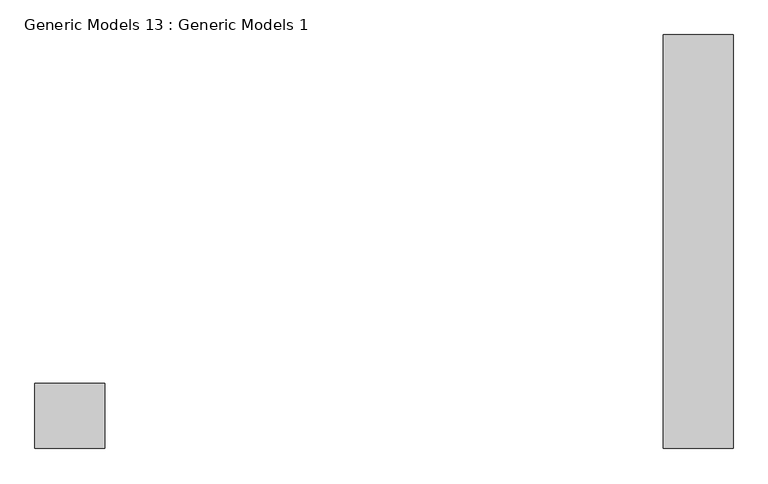
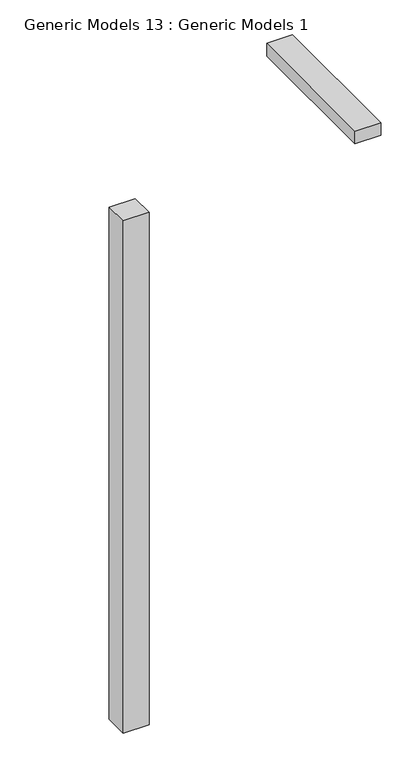
"""IFC4 building model written with IfcOpenShell, lengths in millimetres: proxy geometry, Generic Models 13 : Generic Models 1."""

from ifc_helpers import new_model, si_unit, frame, origin, origin_with_axes, place, context, project, spatial, polyline, outline, extrude, source, transform, mapped, element, save


def generic_models_13_generic_models_1_8ceb580d(model_context):
    return source(origin(), model_context, "Body", "SweptSolid", [
        extrude(outline(polyline([(-9698.5642415, -4709.7273102), (-9546.1642415, -4709.7273102), (-9546.1642415, -5613.7098142), (-9698.5642415, -5613.7098142), (-9698.5642415, -4709.7273102)])), frame((0.0, 0.0, 3200.4), z_axis=(0.0, 0.0, 1.0), x_axis=(1.0, 0.0, 0.0)), (0.0, 0.0, 1.0), 79.9931522),
        extrude(outline(polyline([(-11070.9010638, -5471.7273102), (-10918.5010638, -5471.7273102), (-10918.5010638, -5613.7098142), (-11070.9010638, -5613.7098142), (-11070.9010638, -5471.7273102)])), origin_with_axes(), (0.0, 0.0, 1.0), 3200.4),
    ])


if __name__ == "__main__":
    model = new_model("IFC4")
    model_context = context("Model", 3, world=origin())
    ifc_project = project(units=[si_unit("LENGTHUNIT", "METRE", prefix="MILLI")], contexts=[model_context])
    site = spatial("IfcSite", under=ifc_project)
    building = spatial("IfcBuilding", under=site)
    placement = place(None, origin())
    generic_models_13_generic_models_1_shape = generic_models_13_generic_models_1_8ceb580d(model_context)
    element("IfcBuildingElementProxy", 1, Name="Generic Models 13 : Generic Models 1", ObjectType="Generic Models 13 : Generic Models 1", at=placement, inside=building, context=model_context, shape_type="MappedRepresentation", body=[
        mapped(generic_models_13_generic_models_1_shape, transform((0.0, 0.0, 0.0), x_axis=(1.0, 0.0, 0.0), y_axis=(0.0, 1.0, 0.0), z_axis=(0.0, 0.0, 1.0))),
    ])
    save(model, "model.ifc")
